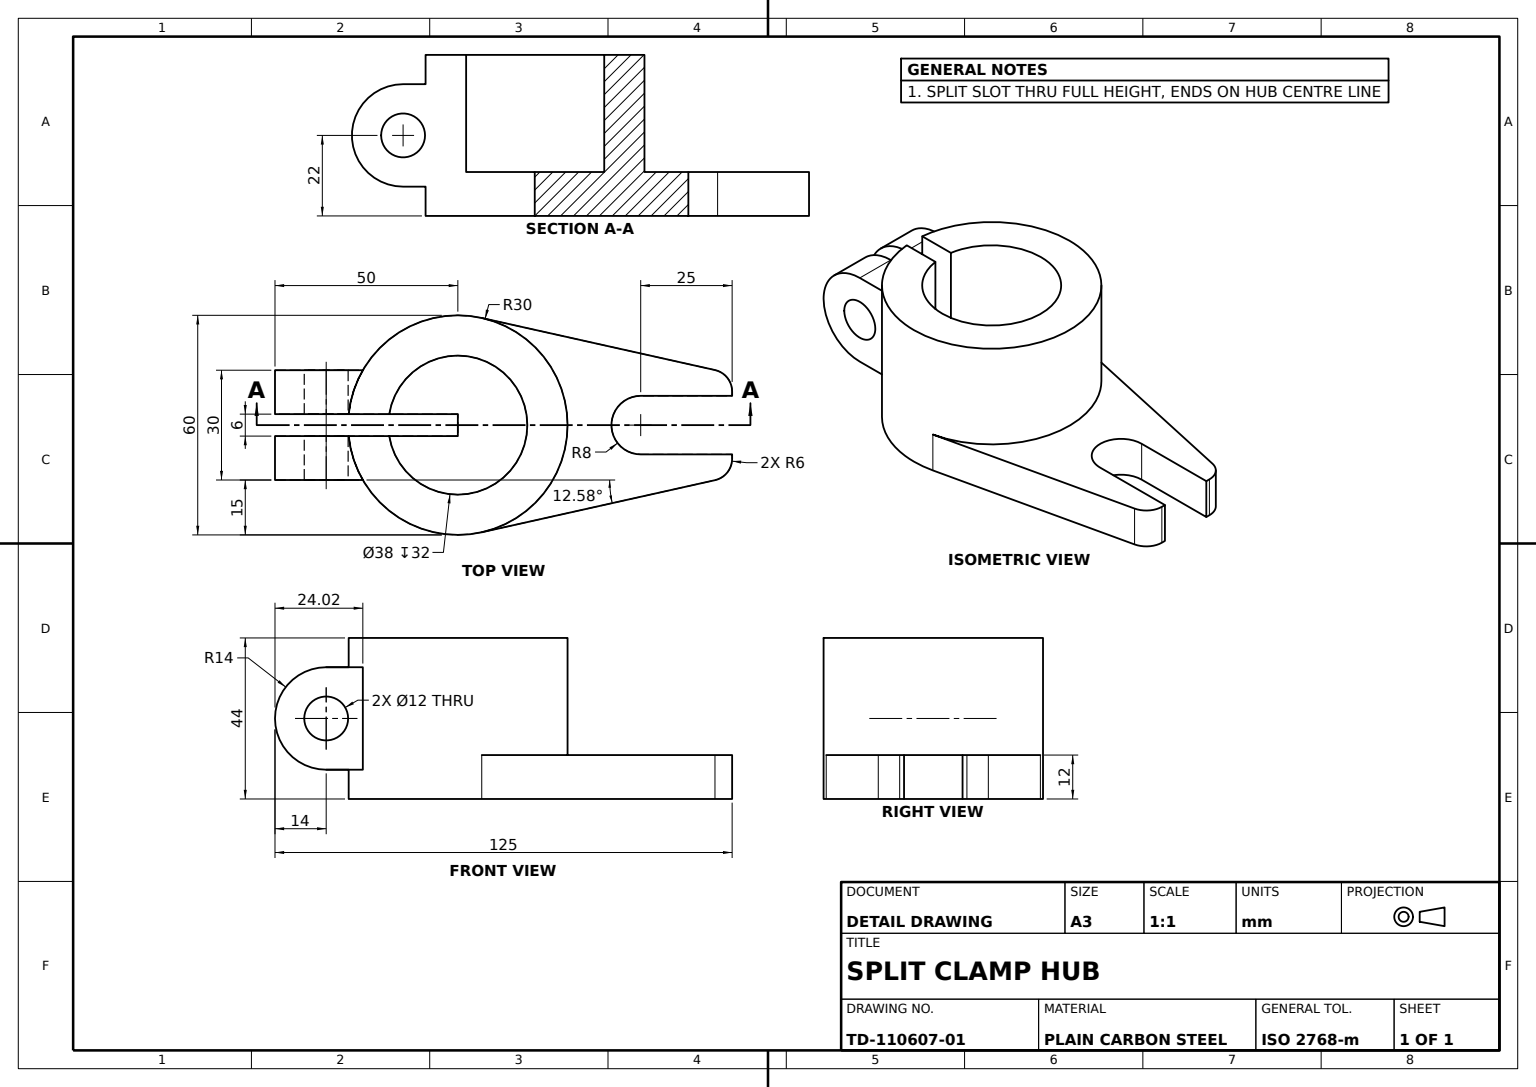
SolidWorks part; units mm, degrees
material "Plain Carbon Steel"
ref_plane "Front Plane" through (0, 0, 0) normal (0, 0, 1) x (1, 0, 0)
ref_plane "Top Plane" through (0, 0, 0) normal (0, 1, 0) x (1, 0, 0)
ref_plane "Right Plane" through (0, 0, 0) normal (1, 0, 0) x (0, 0, -1)
sketch "Base Flange Sketch" plane through (0, 0, 0) normal (0, 1, 0) x (1, 0, 0)
  line L0 (0, 3) -> (0, -3)
  line L1 (-30, -3) -> (0, -3)
  line L2 (-30, 3) -> (0, 3)
  line L3 (75, -9.1914) -> (75, -8)
  line L4 (50, -8) -> (75, -8)
  line L5 (50, 8) -> (75, 8)
  line L6 (6.5345, -29.2797) -> (70.3069, -15.0474)
  line L8 (6.5345, 29.2797) -> (70.3069, 15.0474)
  line L9 (75, 8) -> (75, 9.1914)
  arc A0 (-29.8496, -3) -> (6.5345, -29.2797) centre (0, 0) ccw
  arc A1 (50, 8) -> (50, -8) centre (50, 0) ccw
  arc A2 (75, -9.1914) -> (70.3069, -15.0474) centre (69, -9.1914) cw
  arc A3 (75, 9.1914) -> (70.3069, 15.0474) centre (69, 9.1914) ccw
  arc A4 (6.5345, 29.2797) -> (-29.8496, 3) centre (0, 0) ccw
  point P10 (75, 0)
  point P18 (75, 0)
  point P20 (75, 0)
  dimension "D1" = 60
  dimension "D5" = 50
  dimension "D6" = 6
  dimension "D7" = 6
  dimension "D2" = 6
  dimension "D3" = 30
  dimension "D4" = 3
  dimension "D8" = 25
  dimension "D9" = 75
  dimension "D10" = 16
  dimension "D11" = 1.1914
extrude "Base Flange" add sketch "Base Flange Sketch" along normal blind 12 contours L8 A4 L2 L0 L1 A0 L6 A2 L3 L4 A1 L5 L9 A3
sketch "Clamp Ring Sketch" plane through (0, 12, 0) normal (0, 1, 0) x (1, 0, 0)
  line L0 (-29.8496, 3) -> (0, 3)
  line L1 (0, 3) -> (0, -3)
  line L2 (0, -3) -> (-29.8496, -3)
  arc A0 (-29.8496, -3) -> (-29.8496, 3) centre (0, 0) ccw
  arc A1 (-18.7617, -3) -> (-18.7617, 3) centre (0, 0) ccw
  arc M2 (6.5345, 29.2797) -> (-29.8496, 3) centre (0, 0) ccw
  line M3 (-29.8496, 3) -> (0, 3)
  arc M6 (-29.8496, -3) -> (6.5345, -29.2797) centre (0, 0) ccw
  dimension "D1" = 19
extrude "Split Clamp Ring" add sketch "Clamp Ring Sketch" along normal blind 32 contours A1 L2 A0 M6 M2 M3
ref_plane "Clamp Ear A Plane" through (0, 0, 3) normal (0, 0, 1) x (1, 0, 0)
sketch "Clamp Ear A Sketch" plane through (0, 0, 3) normal (0, 0, 1) x (1, 0, 0)
  line L0 (-36, 36) -> (-25, 36)
  line L1 (-25, 36) -> (-25, 8)
  line L2 (-25, 8) -> (-36, 8)
  arc A1 (-36, 36) -> (-36, 8) centre (-36, 22) ccw
  circle A2 centre (-36, 22) radius 6
  dimension "D1" = 36
  dimension "D3" = 28
  dimension "D4" = 12
  dimension "D2" = 22
  dimension "D5" = 11
extrude "Clamp Ear A" add sketch "Clamp Ear A Sketch" along normal blind 12
ref_plane "Clamp Ear B Plane" through (0, 0, -3) normal (0, 0, 1) x (1, 0, 0)
sketch "Clamp Ear B Sketch" plane through (0, 0, -3) normal (0, 0, 1) x (1, 0, 0)
  line L0 (-36, 36) -> (-25, 36)
  line L1 (-25, 36) -> (-25, 8)
  line L2 (-25, 8) -> (-36, 8)
  arc A0 (-36, 36) -> (-36, 8) centre (-36, 22) ccw
  circle A1 centre (-36, 22) radius 6
  dimension "D1" = 12
  dimension "D2" = 11
extrude "Clamp Ear B" add sketch "Clamp Ear B Sketch" against normal blind 12
